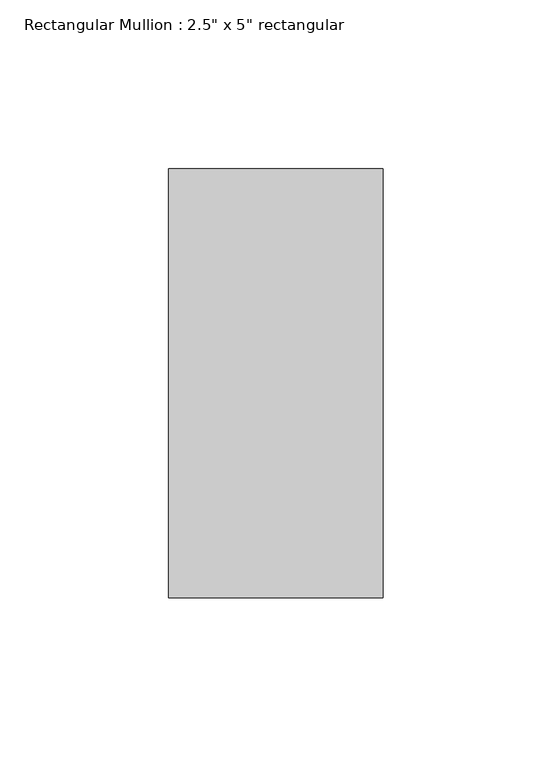
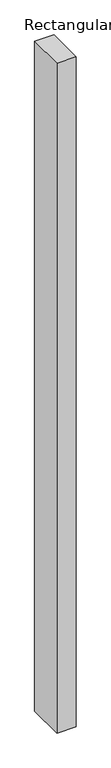
"""IFC4 building model written with IfcOpenShell, lengths in millimetres: member geometry."""

from ifc_helpers import new_model, si_unit, frame, origin, place, context, project, spatial, polyline, outline, extrude, source, transform, mapped, element, save


def member_def95f85(model_context):
    return source(origin(), model_context, "Body", "SweptSolid", [
        extrude(outline(polyline([(31.75, 63.5), (31.75, -63.5), (-31.75, -63.5), (-31.75, 63.5), (31.75, 63.5)])), frame((0.0, 0.0, -2336.8), z_axis=(0.0, 0.0, 1.0), x_axis=(1.0, 0.0, 0.0)), (0.0, 0.0, 1.0), 2336.8),
    ])


if __name__ == "__main__":
    model = new_model("IFC4")
    model_context = context("Model", 3, world=origin())
    ifc_project = project(units=[si_unit("LENGTHUNIT", "METRE", prefix="MILLI")], contexts=[model_context])
    site = spatial("IfcSite", under=ifc_project)
    building = spatial("IfcBuilding", under=site)
    placement = place(None, origin())
    member_shape = member_def95f85(model_context)
    element("IfcMember", 1, ObjectType="Rectangular Mullion : 2.5\" x 5\" rectangular", at=placement, inside=building, context=model_context, shape_type="MappedRepresentation", body=[
        mapped(member_shape, transform((0.0, 0.0, 0.0), x_axis=(1.0, 0.0, 0.0), y_axis=(0.0, 1.0, 0.0), z_axis=(0.0, 0.0, 1.0))),
    ])
    save(model, "model.ifc")

# Revit data of these elements
# Type "Rectangular Mullion : 2.5\" x 5\" rectangular"
#   built-in parameter 1007304 = 0.416667 (stored number, unit not read)
#   built-in parameter 1007301 = 0.104167 (stored number, unit not read)
#   built-in parameter 1007300 = 0.104167 (stored number, unit not read)
# Element 1 (IfcMember, "Rectangular Mullion : 2.5\" x 5\" rectangular")
#   Materials on its faces: "Aluminum"
# Materials
#   "Aluminum": class "Metal", colour RGB 247 247 247, transparency 0, Description = "Aluminum 6061", Cost = 0
